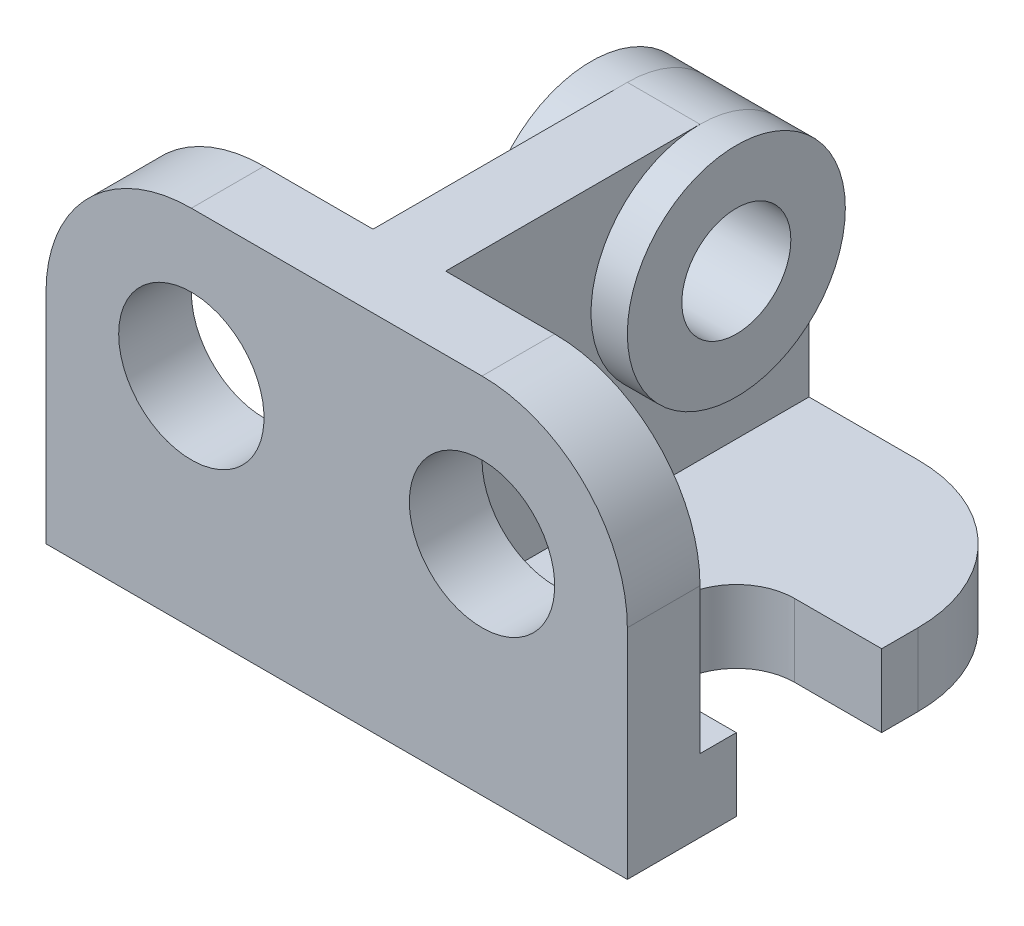
ISO-10303-21;
HEADER;
FILE_DESCRIPTION(('STEP AP214'),'2;1');
FILE_NAME('part.step','',(''),(''),'','','');
FILE_SCHEMA(('AUTOMOTIVE_DESIGN { 1 0 10303 214 1 1 1 1 }'));
ENDSEC;
DATA;
#1=APPLICATION_CONTEXT('core data for automotive mechanical design processes');
#2=APPLICATION_PROTOCOL_DEFINITION('international standard','automotive_design',2000,#1);
#3=PRODUCT_CONTEXT('',#1,'mechanical');
#4=PRODUCT('Part','Part','',(#3));
#5=PRODUCT_RELATED_PRODUCT_CATEGORY('part','',(#4));
#6=PRODUCT_DEFINITION_FORMATION('','',#4);
#7=PRODUCT_DEFINITION_CONTEXT('part definition',#1,'design');
#8=PRODUCT_DEFINITION('design','',#6,#7);
#9=PRODUCT_DEFINITION_SHAPE('','',#8);
#10=(LENGTH_UNIT() NAMED_UNIT(*) SI_UNIT(.MILLI.,.METRE.));
#11=(NAMED_UNIT(*) PLANE_ANGLE_UNIT() SI_UNIT($,.RADIAN.));
#12=(NAMED_UNIT(*) SI_UNIT($,.STERADIAN.) SOLID_ANGLE_UNIT());
#13=UNCERTAINTY_MEASURE_WITH_UNIT(LENGTH_MEASURE(1.E-05),#10,'distance_accuracy_value','');
#14=(GEOMETRIC_REPRESENTATION_CONTEXT(3) GLOBAL_UNCERTAINTY_ASSIGNED_CONTEXT((#13)) GLOBAL_UNIT_ASSIGNED_CONTEXT((#10,
#11,#12)) REPRESENTATION_CONTEXT('',''));
#15=CARTESIAN_POINT('',(0.,0.,0.));
#16=DIRECTION('',(0.,0.,1.));
#17=DIRECTION('',(1.,0.,0.));
#18=AXIS2_PLACEMENT_3D('',#15,#16,#17);
#19=CARTESIAN_POINT('',(4000.,0.,0.));
#20=DIRECTION('',(1.,0.,0.));
#21=DIRECTION('',(0.,0.,-1.));
#22=AXIS2_PLACEMENT_3D('',#19,#20,#21);
#23=PLANE('',#22);
#24=DIRECTION('',(0.,-1.,0.));
#25=VECTOR('',#24,1.);
#26=CARTESIAN_POINT('',(4000.,0.,1500.));
#27=LINE('',#26,#25);
#28=CARTESIAN_POINT('',(4000.,500.,1500.));
#29=VERTEX_POINT('',#28);
#30=CARTESIAN_POINT('',(4000.,-500.,1500.));
#31=VERTEX_POINT('',#30);
#32=EDGE_CURVE('E222',#29,#31,#27,.T.);
#33=ORIENTED_EDGE('',*,*,#32,.F.);
#34=DIRECTION('',(0.,0.,1.));
#35=VECTOR('',#34,1.);
#36=CARTESIAN_POINT('',(4000.,500.,2000.));
#37=LINE('',#36,#35);
#38=CARTESIAN_POINT('',(4000.,500.,2000.));
#39=VERTEX_POINT('',#38);
#40=EDGE_CURVE('E238',#29,#39,#37,.T.);
#41=ORIENTED_EDGE('',*,*,#40,.T.);
#42=DIRECTION('',(0.,1.,0.));
#43=VECTOR('',#42,1.);
#44=CARTESIAN_POINT('',(4000.,500.,2000.));
#45=LINE('',#44,#43);
#46=CARTESIAN_POINT('',(4000.,2500.,2000.));
#47=VERTEX_POINT('',#46);
#48=EDGE_CURVE('E240',#39,#47,#45,.T.);
#49=ORIENTED_EDGE('',*,*,#48,.T.);
#50=DIRECTION('',(0.,0.,1.));
#51=VECTOR('',#50,1.);
#52=CARTESIAN_POINT('',(4000.,2500.,3000.));
#53=LINE('',#52,#51);
#54=CARTESIAN_POINT('',(4000.,2500.,3000.));
#55=VERTEX_POINT('',#54);
#56=EDGE_CURVE('E285',#47,#55,#53,.T.);
#57=ORIENTED_EDGE('',*,*,#56,.T.);
#58=DIRECTION('',(0.,-1.,0.));
#59=VECTOR('',#58,1.);
#60=CARTESIAN_POINT('',(4000.,500.,3000.));
#61=LINE('',#60,#59);
#62=CARTESIAN_POINT('',(4000.,-500.,3000.));
#63=VERTEX_POINT('',#62);
#64=EDGE_CURVE('E241',#55,#63,#61,.T.);
#65=ORIENTED_EDGE('',*,*,#64,.T.);
#66=DIRECTION('',(0.,0.,-1.));
#67=VECTOR('',#66,1.);
#68=CARTESIAN_POINT('',(4000.,-500.,3000.));
#69=LINE('',#68,#67);
#70=EDGE_CURVE('E249',#63,#31,#69,.T.);
#71=ORIENTED_EDGE('',*,*,#70,.T.);
#72=EDGE_LOOP('',(#33,#41,#49,#57,#65,#71));
#73=FACE_BOUND('',#72,.T.);
#74=ADVANCED_FACE('F41',(#73),#23,.T.);
#75=CARTESIAN_POINT('',(-4000.,0.,0.));
#76=DIRECTION('',(1.,0.,0.));
#77=DIRECTION('',(0.,0.,-1.));
#78=AXIS2_PLACEMENT_3D('',#75,#76,#77);
#79=PLANE('',#78);
#80=DIRECTION('',(0.,0.,1.));
#81=VECTOR('',#80,1.);
#82=CARTESIAN_POINT('',(-4000.,500.,2000.));
#83=LINE('',#82,#81);
#84=CARTESIAN_POINT('',(-4000.,500.,1447.76070932594));
#85=VERTEX_POINT('',#84);
#86=CARTESIAN_POINT('',(-4000.,500.,2000.));
#87=VERTEX_POINT('',#86);
#88=EDGE_CURVE('E257',#85,#87,#83,.T.);
#89=ORIENTED_EDGE('',*,*,#88,.F.);
#90=DIRECTION('',(0.,-1.,0.));
#91=VECTOR('',#90,1.);
#92=CARTESIAN_POINT('',(-4000.,0.,1447.76070932594));
#93=LINE('',#92,#91);
#94=CARTESIAN_POINT('',(-4000.,-500.,1447.76070932594));
#95=VERTEX_POINT('',#94);
#96=EDGE_CURVE('E341',#85,#95,#93,.T.);
#97=ORIENTED_EDGE('',*,*,#96,.T.);
#98=DIRECTION('',(0.,0.,-1.));
#99=VECTOR('',#98,1.);
#100=CARTESIAN_POINT('',(-4000.,-500.,3000.));
#101=LINE('',#100,#99);
#102=CARTESIAN_POINT('',(-4000.,-500.,3000.));
#103=VERTEX_POINT('',#102);
#104=EDGE_CURVE('E243',#103,#95,#101,.T.);
#105=ORIENTED_EDGE('',*,*,#104,.F.);
#106=DIRECTION('',(0.,-1.,0.));
#107=VECTOR('',#106,1.);
#108=CARTESIAN_POINT('',(-4000.,500.,3000.));
#109=LINE('',#108,#107);
#110=CARTESIAN_POINT('',(-4000.,2500.,3000.));
#111=VERTEX_POINT('',#110);
#112=EDGE_CURVE('E263',#111,#103,#109,.T.);
#113=ORIENTED_EDGE('',*,*,#112,.F.);
#114=DIRECTION('',(0.,0.,1.));
#115=VECTOR('',#114,1.);
#116=CARTESIAN_POINT('',(-4000.,2500.,0.));
#117=LINE('',#116,#115);
#118=CARTESIAN_POINT('',(-4000.,2500.,2000.));
#119=VERTEX_POINT('',#118);
#120=EDGE_CURVE('E304',#111,#119,#117,.F.);
#121=ORIENTED_EDGE('',*,*,#120,.T.);
#122=DIRECTION('',(0.,1.,0.));
#123=VECTOR('',#122,1.);
#124=CARTESIAN_POINT('',(-4000.,500.,2000.));
#125=LINE('',#124,#123);
#126=EDGE_CURVE('E260',#87,#119,#125,.T.);
#127=ORIENTED_EDGE('',*,*,#126,.F.);
#128=EDGE_LOOP('',(#89,#97,#105,#113,#121,#127));
#129=FACE_BOUND('',#128,.T.);
#130=ADVANCED_FACE('F519',(#129),#79,.F.);
#131=CARTESIAN_POINT('',(500.,-500.,-3000.));
#132=DIRECTION('',(1.,0.,0.));
#133=DIRECTION('',(0.,0.,-1.));
#134=AXIS2_PLACEMENT_3D('',#131,#132,#133);
#135=PLANE('',#134);
#136=DIRECTION('',(0.,1.,0.));
#137=VECTOR('',#136,1.);
#138=CARTESIAN_POINT('',(500.,-500.,-3000.));
#139=LINE('',#138,#137);
#140=CARTESIAN_POINT('',(500.,500.,-3000.));
#141=VERTEX_POINT('',#140);
#142=CARTESIAN_POINT('',(500.,3000.,-3000.));
#143=VERTEX_POINT('',#142);
#144=EDGE_CURVE('E431',#141,#143,#139,.T.);
#145=ORIENTED_EDGE('',*,*,#144,.T.);
#146=CARTESIAN_POINT('',(500.,3000.,-1500.));
#147=DIRECTION('',(1.,0.,0.));
#148=DIRECTION('',(0.,0.,-1.));
#149=AXIS2_PLACEMENT_3D('',#146,#147,#148);
#150=CIRCLE('',#149,1500.);
#151=CARTESIAN_POINT('',(500.,4500.,-1500.));
#152=VERTEX_POINT('',#151);
#153=EDGE_CURVE('E335',#143,#152,#150,.F.);
#154=ORIENTED_EDGE('',*,*,#153,.T.);
#155=DIRECTION('',(0.,0.,-1.));
#156=VECTOR('',#155,1.);
#157=CARTESIAN_POINT('',(500.,4500.,-3000.));
#158=LINE('',#157,#156);
#159=CARTESIAN_POINT('',(500.,4500.,2000.));
#160=VERTEX_POINT('',#159);
#161=EDGE_CURVE('E426',#160,#152,#158,.T.);
#162=ORIENTED_EDGE('',*,*,#161,.F.);
#163=DIRECTION('',(0.,1.,0.));
#164=VECTOR('',#163,1.);
#165=CARTESIAN_POINT('',(500.,500.,2000.));
#166=LINE('',#165,#164);
#167=CARTESIAN_POINT('',(500.,500.,2000.));
#168=VERTEX_POINT('',#167);
#169=EDGE_CURVE('E434',#168,#160,#166,.T.);
#170=ORIENTED_EDGE('',*,*,#169,.F.);
#171=DIRECTION('',(0.,0.,1.));
#172=VECTOR('',#171,1.);
#173=CARTESIAN_POINT('',(500.,500.,2000.));
#174=LINE('',#173,#172);
#175=EDGE_CURVE('E439',#141,#168,#174,.T.);
#176=ORIENTED_EDGE('',*,*,#175,.F.);
#177=EDGE_LOOP('',(#145,#154,#162,#170,#176));
#178=FACE_BOUND('',#177,.T.);
#179=ADVANCED_FACE('F555',(#178),#135,.T.);
#180=CARTESIAN_POINT('',(4000.,500.,2000.));
#181=DIRECTION('',(0.,-1.,0.));
#182=DIRECTION('',(0.,0.,-1.));
#183=AXIS2_PLACEMENT_3D('',#180,#181,#182);
#184=PLANE('',#183);
#185=DIRECTION('',(0.,0.,-1.));
#186=VECTOR('',#185,1.);
#187=CARTESIAN_POINT('',(-2000.,500.,447.760709325942));
#188=LINE('',#187,#186);
#189=CARTESIAN_POINT('',(-2000.,500.,647.760709325942));
#190=VERTEX_POINT('',#189);
#191=CARTESIAN_POINT('',(-2000.,500.,247.760709325942));
#192=VERTEX_POINT('',#191);
#193=EDGE_CURVE('E400',#190,#192,#188,.T.);
#194=ORIENTED_EDGE('',*,*,#193,.F.);
#195=CARTESIAN_POINT('',(-2800.,500.,647.760709325942));
#196=DIRECTION('',(0.,-1.,0.));
#197=DIRECTION('',(0.,0.,-1.));
#198=AXIS2_PLACEMENT_3D('',#195,#196,#197);
#199=CIRCLE('',#198,800.);
#200=CARTESIAN_POINT('',(-2800.,500.,1447.76070932594));
#201=VERTEX_POINT('',#200);
#202=EDGE_CURVE('E355',#190,#201,#199,.T.);
#203=ORIENTED_EDGE('',*,*,#202,.T.);
#204=DIRECTION('',(1.,0.,0.));
#205=VECTOR('',#204,1.);
#206=CARTESIAN_POINT('',(-5200.,500.,1447.76070932594));
#207=LINE('',#206,#205);
#208=EDGE_CURVE('E405',#85,#201,#207,.T.);
#209=ORIENTED_EDGE('',*,*,#208,.F.);
#210=ORIENTED_EDGE('',*,*,#88,.T.);
#211=DIRECTION('',(-1.,0.,0.));
#212=VECTOR('',#211,1.);
#213=CARTESIAN_POINT('',(4000.,500.,2000.));
#214=LINE('',#213,#212);
#215=CARTESIAN_POINT('',(-500.,500.,2000.));
#216=VERTEX_POINT('',#215);
#217=EDGE_CURVE('E276',#216,#87,#214,.T.);
#218=ORIENTED_EDGE('',*,*,#217,.F.);
#219=DIRECTION('',(0.,0.,-1.));
#220=VECTOR('',#219,1.);
#221=CARTESIAN_POINT('',(-500.,500.,2000.));
#222=LINE('',#221,#220);
#223=CARTESIAN_POINT('',(-500.,500.,-3000.));
#224=VERTEX_POINT('',#223);
#225=EDGE_CURVE('E447',#216,#224,#222,.T.);
#226=ORIENTED_EDGE('',*,*,#225,.T.);
#227=DIRECTION('',(-1.,0.,0.));
#228=VECTOR('',#227,1.);
#229=CARTESIAN_POINT('',(4000.,500.,-3000.));
#230=LINE('',#229,#228);
#231=CARTESIAN_POINT('',(-2000.,500.,-3000.));
#232=VERTEX_POINT('',#231);
#233=EDGE_CURVE('E279',#224,#232,#230,.T.);
#234=ORIENTED_EDGE('',*,*,#233,.T.);
#235=CARTESIAN_POINT('',(-2000.,500.,-1000.));
#236=DIRECTION('',(0.,-1.,0.));
#237=DIRECTION('',(0.,0.,-1.));
#238=AXIS2_PLACEMENT_3D('',#235,#236,#237);
#239=CIRCLE('',#238,2000.);
#240=CARTESIAN_POINT('',(-4000.,500.,-1000.));
#241=VERTEX_POINT('',#240);
#242=EDGE_CURVE('E321',#232,#241,#239,.F.);
#243=ORIENTED_EDGE('',*,*,#242,.T.);
#244=CARTESIAN_POINT('',(-4000.,500.,-552.239290674058));
#245=VERTEX_POINT('',#244);
#246=EDGE_CURVE('E251',#241,#245,#83,.T.);
#247=ORIENTED_EDGE('',*,*,#246,.T.);
#248=DIRECTION('',(-1.,0.,0.));
#249=VECTOR('',#248,1.);
#250=CARTESIAN_POINT('',(-5200.,500.,-552.239290674058));
#251=LINE('',#250,#249);
#252=CARTESIAN_POINT('',(-2800.,500.,-552.239290674058));
#253=VERTEX_POINT('',#252);
#254=EDGE_CURVE('E399',#253,#245,#251,.T.);
#255=ORIENTED_EDGE('',*,*,#254,.F.);
#256=CARTESIAN_POINT('',(-2800.,500.,247.760709325942));
#257=DIRECTION('',(0.,-1.,0.));
#258=DIRECTION('',(0.,0.,-1.));
#259=AXIS2_PLACEMENT_3D('',#256,#257,#258);
#260=CIRCLE('',#259,800.);
#261=EDGE_CURVE('E363',#253,#192,#260,.T.);
#262=ORIENTED_EDGE('',*,*,#261,.T.);
#263=EDGE_LOOP('',(#194,#203,#209,#210,#218,#226,#234,#243,#247,#255,#262));
#264=FACE_BOUND('',#263,.T.);
#265=ADVANCED_FACE('F461',(#264),#184,.F.);
#266=CARTESIAN_POINT('',(4000.,500.,2000.));
#267=DIRECTION('',(0.,0.,1.));
#268=DIRECTION('',(1.,0.,0.));
#269=AXIS2_PLACEMENT_3D('',#266,#267,#268);
#270=PLANE('',#269);
#271=CARTESIAN_POINT('',(-2000.,2500.,2000.));
#272=DIRECTION('',(0.,0.,-1.));
#273=DIRECTION('',(-1.,0.,0.));
#274=AXIS2_PLACEMENT_3D('',#271,#272,#273);
#275=CIRCLE('',#274,1000.);
#276=CARTESIAN_POINT('',(-3000.,2500.,2000.));
#277=VERTEX_POINT('',#276);
#278=EDGE_CURVE('E244',#277,#277,#275,.T.);
#279=ORIENTED_EDGE('',*,*,#278,.F.);
#280=EDGE_LOOP('',(#279));
#281=FACE_BOUND('',#280,.T.);
#282=DIRECTION('',(-1.,0.,0.));
#283=VECTOR('',#282,1.);
#284=CARTESIAN_POINT('',(4000.,4500.,2000.));
#285=LINE('',#284,#283);
#286=CARTESIAN_POINT('',(-500.,4500.,2000.));
#287=VERTEX_POINT('',#286);
#288=CARTESIAN_POINT('',(-2000.,4500.,2000.));
#289=VERTEX_POINT('',#288);
#290=EDGE_CURVE('E275',#287,#289,#285,.T.);
#291=ORIENTED_EDGE('',*,*,#290,.F.);
#292=DIRECTION('',(0.,-1.,0.));
#293=VECTOR('',#292,1.);
#294=CARTESIAN_POINT('',(-500.,500.,2000.));
#295=LINE('',#294,#293);
#296=EDGE_CURVE('E442',#287,#216,#295,.T.);
#297=ORIENTED_EDGE('',*,*,#296,.T.);
#298=ORIENTED_EDGE('',*,*,#217,.T.);
#299=ORIENTED_EDGE('',*,*,#126,.T.);
#300=CARTESIAN_POINT('',(-2000.,2500.,2000.));
#301=DIRECTION('',(0.,0.,1.));
#302=DIRECTION('',(1.,0.,0.));
#303=AXIS2_PLACEMENT_3D('',#300,#301,#302);
#304=CIRCLE('',#303,2000.);
#305=EDGE_CURVE('E310',#119,#289,#304,.F.);
#306=ORIENTED_EDGE('',*,*,#305,.T.);
#307=EDGE_LOOP('',(#291,#297,#298,#299,#306));
#308=FACE_BOUND('',#307,.T.);
#309=ADVANCED_FACE('F459',(#281,#308),#270,.F.);
#310=CARTESIAN_POINT('',(4000.,500.,-3000.));
#311=DIRECTION('',(0.,0.,1.));
#312=DIRECTION('',(1.,0.,0.));
#313=AXIS2_PLACEMENT_3D('',#310,#311,#312);
#314=PLANE('',#313);
#315=DIRECTION('',(0.,1.,0.));
#316=VECTOR('',#315,1.);
#317=CARTESIAN_POINT('',(-500.,-500.,-3000.));
#318=LINE('',#317,#316);
#319=CARTESIAN_POINT('',(-500.,3000.,-3000.));
#320=VERTEX_POINT('',#319);
#321=EDGE_CURVE('E435',#224,#320,#318,.T.);
#322=ORIENTED_EDGE('',*,*,#321,.T.);
#323=DIRECTION('',(-1.,0.,0.));
#324=VECTOR('',#323,1.);
#325=CARTESIAN_POINT('',(4000.,3000.,-3000.));
#326=LINE('',#325,#324);
#327=EDGE_CURVE('E337',#320,#143,#326,.F.);
#328=ORIENTED_EDGE('',*,*,#327,.T.);
#329=ORIENTED_EDGE('',*,*,#144,.F.);
#330=CARTESIAN_POINT('',(2000.,500.,-3000.));
#331=VERTEX_POINT('',#330);
#332=EDGE_CURVE('E283',#331,#141,#230,.T.);
#333=ORIENTED_EDGE('',*,*,#332,.F.);
#334=DIRECTION('',(0.,1.,0.));
#335=VECTOR('',#334,1.);
#336=CARTESIAN_POINT('',(2000.,-500.,-3000.));
#337=LINE('',#336,#335);
#338=CARTESIAN_POINT('',(2000.,-500.,-3000.));
#339=VERTEX_POINT('',#338);
#340=EDGE_CURVE('E312',#331,#339,#337,.F.);
#341=ORIENTED_EDGE('',*,*,#340,.T.);
#342=DIRECTION('',(-1.,0.,0.));
#343=VECTOR('',#342,1.);
#344=CARTESIAN_POINT('',(4000.,-500.,-3000.));
#345=LINE('',#344,#343);
#346=CARTESIAN_POINT('',(-2000.,-500.,-3000.));
#347=VERTEX_POINT('',#346);
#348=EDGE_CURVE('E254',#339,#347,#345,.T.);
#349=ORIENTED_EDGE('',*,*,#348,.T.);
#350=DIRECTION('',(0.,1.,0.));
#351=VECTOR('',#350,1.);
#352=CARTESIAN_POINT('',(-2000.,500.,-3000.));
#353=LINE('',#352,#351);
#354=EDGE_CURVE('E319',#347,#232,#353,.T.);
#355=ORIENTED_EDGE('',*,*,#354,.T.);
#356=ORIENTED_EDGE('',*,*,#233,.F.);
#357=EDGE_LOOP('',(#322,#328,#329,#333,#341,#349,#355,#356));
#358=FACE_BOUND('',#357,.T.);
#359=ADVANCED_FACE('F456',(#358),#314,.F.);
#360=ORIENTED_EDGE('',*,*,#40,.F.);
#361=DIRECTION('',(1.,0.,0.));
#362=VECTOR('',#361,1.);
#363=CARTESIAN_POINT('',(2000.,500.,1500.));
#364=LINE('',#363,#362);
#365=CARTESIAN_POINT('',(2800.,500.,1500.));
#366=VERTEX_POINT('',#365);
#367=EDGE_CURVE('E389',#366,#29,#364,.T.);
#368=ORIENTED_EDGE('',*,*,#367,.F.);
#369=CARTESIAN_POINT('',(2800.,500.,700.));
#370=DIRECTION('',(0.,-1.,0.));
#371=DIRECTION('',(0.,0.,-1.));
#372=AXIS2_PLACEMENT_3D('',#369,#370,#371);
#373=CIRCLE('',#372,800.);
#374=CARTESIAN_POINT('',(2000.,500.,700.));
#375=VERTEX_POINT('',#374);
#376=EDGE_CURVE('E372',#366,#375,#373,.T.);
#377=ORIENTED_EDGE('',*,*,#376,.T.);
#378=DIRECTION('',(0.,0.,1.));
#379=VECTOR('',#378,1.);
#380=CARTESIAN_POINT('',(2000.,500.,-500.000000000001));
#381=LINE('',#380,#379);
#382=CARTESIAN_POINT('',(2000.,500.,299.999999999999));
#383=VERTEX_POINT('',#382);
#384=EDGE_CURVE('E233',#383,#375,#381,.T.);
#385=ORIENTED_EDGE('',*,*,#384,.F.);
#386=CARTESIAN_POINT('',(2800.,500.,299.999999999999));
#387=DIRECTION('',(0.,-1.,0.));
#388=DIRECTION('',(0.,0.,-1.));
#389=AXIS2_PLACEMENT_3D('',#386,#387,#388);
#390=CIRCLE('',#389,800.);
#391=CARTESIAN_POINT('',(2800.,500.,-500.000000000001));
#392=VERTEX_POINT('',#391);
#393=EDGE_CURVE('E47',#383,#392,#390,.T.);
#394=ORIENTED_EDGE('',*,*,#393,.T.);
#395=DIRECTION('',(-1.,0.,0.));
#396=VECTOR('',#395,1.);
#397=CARTESIAN_POINT('',(2000.,500.,-500.000000000001));
#398=LINE('',#397,#396);
#399=CARTESIAN_POINT('',(4000.,500.,-500.000000000001));
#400=VERTEX_POINT('',#399);
#401=EDGE_CURVE('E220',#400,#392,#398,.T.);
#402=ORIENTED_EDGE('',*,*,#401,.F.);
#403=CARTESIAN_POINT('',(4000.,500.,-1000.));
#404=VERTEX_POINT('',#403);
#405=EDGE_CURVE('E229',#404,#400,#37,.T.);
#406=ORIENTED_EDGE('',*,*,#405,.F.);
#407=CARTESIAN_POINT('',(2000.,500.,-1000.));
#408=DIRECTION('',(0.,-1.,0.));
#409=DIRECTION('',(0.,0.,-1.));
#410=AXIS2_PLACEMENT_3D('',#407,#408,#409);
#411=CIRCLE('',#410,2000.);
#412=EDGE_CURVE('E311',#404,#331,#411,.F.);
#413=ORIENTED_EDGE('',*,*,#412,.T.);
#414=ORIENTED_EDGE('',*,*,#332,.T.);
#415=ORIENTED_EDGE('',*,*,#175,.T.);
#416=EDGE_CURVE('E280',#39,#168,#214,.T.);
#417=ORIENTED_EDGE('',*,*,#416,.F.);
#418=EDGE_LOOP('',(#360,#368,#377,#385,#394,#402,#406,#413,#414,#415,#417));
#419=FACE_BOUND('',#418,.T.);
#420=ADVANCED_FACE('F230',(#419),#184,.F.);
#421=CARTESIAN_POINT('',(2000.,2500.,2000.));
#422=DIRECTION('',(0.,0.,-1.));
#423=DIRECTION('',(-1.,0.,0.));
#424=AXIS2_PLACEMENT_3D('',#421,#422,#423);
#425=CIRCLE('',#424,1000.);
#426=CARTESIAN_POINT('',(1000.,2500.,2000.));
#427=VERTEX_POINT('',#426);
#428=EDGE_CURVE('E287',#427,#427,#425,.T.);
#429=ORIENTED_EDGE('',*,*,#428,.F.);
#430=EDGE_LOOP('',(#429));
#431=FACE_BOUND('',#430,.T.);
#432=ORIENTED_EDGE('',*,*,#416,.T.);
#433=ORIENTED_EDGE('',*,*,#169,.T.);
#434=CARTESIAN_POINT('',(2000.,4500.,2000.));
#435=VERTEX_POINT('',#434);
#436=EDGE_CURVE('E271',#435,#160,#285,.T.);
#437=ORIENTED_EDGE('',*,*,#436,.F.);
#438=CARTESIAN_POINT('',(2000.,2500.,2000.));
#439=DIRECTION('',(0.,0.,1.));
#440=DIRECTION('',(1.,0.,0.));
#441=AXIS2_PLACEMENT_3D('',#438,#439,#440);
#442=CIRCLE('',#441,2000.);
#443=EDGE_CURVE('E296',#435,#47,#442,.F.);
#444=ORIENTED_EDGE('',*,*,#443,.T.);
#445=ORIENTED_EDGE('',*,*,#48,.F.);
#446=EDGE_LOOP('',(#432,#433,#437,#444,#445));
#447=FACE_BOUND('',#446,.T.);
#448=ADVANCED_FACE('F463',(#431,#447),#270,.F.);
#449=CARTESIAN_POINT('',(4000.,4500.,3000.));
#450=DIRECTION('',(0.,-1.,0.));
#451=DIRECTION('',(0.,0.,-1.));
#452=AXIS2_PLACEMENT_3D('',#449,#450,#451);
#453=PLANE('',#452);
#454=ORIENTED_EDGE('',*,*,#161,.T.);
#455=DIRECTION('',(-1.,0.,0.));
#456=VECTOR('',#455,1.);
#457=CARTESIAN_POINT('',(4000.,4500.,-1500.));
#458=LINE('',#457,#456);
#459=CARTESIAN_POINT('',(-500.,4500.,-1500.));
#460=VERTEX_POINT('',#459);
#461=EDGE_CURVE('E333',#152,#460,#458,.T.);
#462=ORIENTED_EDGE('',*,*,#461,.T.);
#463=DIRECTION('',(0.,0.,1.));
#464=VECTOR('',#463,1.);
#465=CARTESIAN_POINT('',(-500.,4500.,-3000.));
#466=LINE('',#465,#464);
#467=EDGE_CURVE('E428',#460,#287,#466,.T.);
#468=ORIENTED_EDGE('',*,*,#467,.T.);
#469=ORIENTED_EDGE('',*,*,#290,.T.);
#470=DIRECTION('',(0.,0.,1.));
#471=VECTOR('',#470,1.);
#472=CARTESIAN_POINT('',(-2000.,4500.,3000.));
#473=LINE('',#472,#471);
#474=CARTESIAN_POINT('',(-2000.,4500.,3000.));
#475=VERTEX_POINT('',#474);
#476=EDGE_CURVE('E297',#289,#475,#473,.T.);
#477=ORIENTED_EDGE('',*,*,#476,.T.);
#478=DIRECTION('',(-1.,0.,0.));
#479=VECTOR('',#478,1.);
#480=CARTESIAN_POINT('',(4000.,4500.,3000.));
#481=LINE('',#480,#479);
#482=CARTESIAN_POINT('',(2000.,4500.,3000.));
#483=VERTEX_POINT('',#482);
#484=EDGE_CURVE('E269',#483,#475,#481,.T.);
#485=ORIENTED_EDGE('',*,*,#484,.F.);
#486=DIRECTION('',(0.,0.,1.));
#487=VECTOR('',#486,1.);
#488=CARTESIAN_POINT('',(2000.,4500.,2000.));
#489=LINE('',#488,#487);
#490=EDGE_CURVE('E298',#483,#435,#489,.F.);
#491=ORIENTED_EDGE('',*,*,#490,.T.);
#492=ORIENTED_EDGE('',*,*,#436,.T.);
#493=EDGE_LOOP('',(#454,#462,#468,#469,#477,#485,#491,#492));
#494=FACE_BOUND('',#493,.T.);
#495=ADVANCED_FACE('F471',(#494),#453,.F.);
#496=CARTESIAN_POINT('',(4000.,500.,3000.));
#497=DIRECTION('',(0.,0.,-1.));
#498=DIRECTION('',(-1.,0.,0.));
#499=AXIS2_PLACEMENT_3D('',#496,#497,#498);
#500=PLANE('',#499);
#501=CARTESIAN_POINT('',(2000.,2500.,3000.));
#502=DIRECTION('',(0.,0.,-1.));
#503=DIRECTION('',(-1.,0.,0.));
#504=AXIS2_PLACEMENT_3D('',#501,#502,#503);
#505=CIRCLE('',#504,1000.);
#506=CARTESIAN_POINT('',(1000.,2500.,3000.));
#507=VERTEX_POINT('',#506);
#508=EDGE_CURVE('E288',#507,#507,#505,.T.);
#509=ORIENTED_EDGE('',*,*,#508,.T.);
#510=EDGE_LOOP('',(#509));
#511=FACE_BOUND('',#510,.T.);
#512=ORIENTED_EDGE('',*,*,#484,.T.);
#513=CARTESIAN_POINT('',(-2000.,2500.,3000.));
#514=DIRECTION('',(0.,0.,-1.));
#515=DIRECTION('',(-1.,0.,0.));
#516=AXIS2_PLACEMENT_3D('',#513,#514,#515);
#517=CIRCLE('',#516,2000.);
#518=EDGE_CURVE('E303',#475,#111,#517,.F.);
#519=ORIENTED_EDGE('',*,*,#518,.T.);
#520=ORIENTED_EDGE('',*,*,#112,.T.);
#521=DIRECTION('',(-1.,0.,0.));
#522=VECTOR('',#521,1.);
#523=CARTESIAN_POINT('',(4000.,-500.,3000.));
#524=LINE('',#523,#522);
#525=EDGE_CURVE('E268',#63,#103,#524,.T.);
#526=ORIENTED_EDGE('',*,*,#525,.F.);
#527=ORIENTED_EDGE('',*,*,#64,.F.);
#528=CARTESIAN_POINT('',(2000.,2500.,3000.));
#529=DIRECTION('',(0.,0.,-1.));
#530=DIRECTION('',(-1.,0.,0.));
#531=AXIS2_PLACEMENT_3D('',#528,#529,#530);
#532=CIRCLE('',#531,2000.);
#533=EDGE_CURVE('E295',#55,#483,#532,.F.);
#534=ORIENTED_EDGE('',*,*,#533,.T.);
#535=EDGE_LOOP('',(#512,#519,#520,#526,#527,#534));
#536=FACE_BOUND('',#535,.T.);
#537=CARTESIAN_POINT('',(-2000.,2500.,3000.));
#538=DIRECTION('',(0.,0.,-1.));
#539=DIRECTION('',(-1.,0.,0.));
#540=AXIS2_PLACEMENT_3D('',#537,#538,#539);
#541=CIRCLE('',#540,1000.);
#542=CARTESIAN_POINT('',(-3000.,2500.,3000.));
#543=VERTEX_POINT('',#542);
#544=EDGE_CURVE('E281',#543,#543,#541,.T.);
#545=ORIENTED_EDGE('',*,*,#544,.T.);
#546=EDGE_LOOP('',(#545));
#547=FACE_BOUND('',#546,.T.);
#548=ADVANCED_FACE('F530',(#511,#536,#547),#500,.F.);
#549=CARTESIAN_POINT('',(4000.,-500.,3000.));
#550=DIRECTION('',(0.,1.,0.));
#551=DIRECTION('',(0.,0.,1.));
#552=AXIS2_PLACEMENT_3D('',#549,#550,#551);
#553=PLANE('',#552);
#554=DIRECTION('',(-1.,0.,0.));
#555=VECTOR('',#554,1.);
#556=CARTESIAN_POINT('',(4000.,-500.,-500.));
#557=LINE('',#556,#555);
#558=CARTESIAN_POINT('',(4000.,-500.,-500.));
#559=VERTEX_POINT('',#558);
#560=CARTESIAN_POINT('',(2800.,-500.,-500.));
#561=VERTEX_POINT('',#560);
#562=EDGE_CURVE('E216',#559,#561,#557,.T.);
#563=ORIENTED_EDGE('',*,*,#562,.T.);
#564=CARTESIAN_POINT('',(2800.,-500.,299.999999999999));
#565=DIRECTION('',(0.,1.,0.));
#566=DIRECTION('',(0.,0.,1.));
#567=AXIS2_PLACEMENT_3D('',#564,#565,#566);
#568=CIRCLE('',#567,800.);
#569=CARTESIAN_POINT('',(2000.,-500.,299.999999999999));
#570=VERTEX_POINT('',#569);
#571=EDGE_CURVE('E11',#561,#570,#568,.T.);
#572=ORIENTED_EDGE('',*,*,#571,.T.);
#573=DIRECTION('',(0.,0.,1.));
#574=VECTOR('',#573,1.);
#575=CARTESIAN_POINT('',(2000.,-500.,3000.));
#576=LINE('',#575,#574);
#577=CARTESIAN_POINT('',(2000.,-500.,700.));
#578=VERTEX_POINT('',#577);
#579=EDGE_CURVE('E366',#570,#578,#576,.T.);
#580=ORIENTED_EDGE('',*,*,#579,.T.);
#581=CARTESIAN_POINT('',(2800.,-500.,700.));
#582=DIRECTION('',(0.,1.,0.));
#583=DIRECTION('',(0.,0.,1.));
#584=AXIS2_PLACEMENT_3D('',#581,#582,#583);
#585=CIRCLE('',#584,800.);
#586=CARTESIAN_POINT('',(2800.,-500.,1500.));
#587=VERTEX_POINT('',#586);
#588=EDGE_CURVE('E380',#578,#587,#585,.T.);
#589=ORIENTED_EDGE('',*,*,#588,.T.);
#590=DIRECTION('',(1.,0.,0.));
#591=VECTOR('',#590,1.);
#592=CARTESIAN_POINT('',(4000.,-500.,1500.));
#593=LINE('',#592,#591);
#594=EDGE_CURVE('E391',#587,#31,#593,.T.);
#595=ORIENTED_EDGE('',*,*,#594,.T.);
#596=ORIENTED_EDGE('',*,*,#70,.F.);
#597=ORIENTED_EDGE('',*,*,#525,.T.);
#598=ORIENTED_EDGE('',*,*,#104,.T.);
#599=DIRECTION('',(1.,0.,0.));
#600=VECTOR('',#599,1.);
#601=CARTESIAN_POINT('',(4000.,-500.,1447.76070932594));
#602=LINE('',#601,#600);
#603=CARTESIAN_POINT('',(-2800.,-500.,1447.76070932594));
#604=VERTEX_POINT('',#603);
#605=EDGE_CURVE('E410',#95,#604,#602,.T.);
#606=ORIENTED_EDGE('',*,*,#605,.T.);
#607=CARTESIAN_POINT('',(-2800.,-500.,647.760709325942));
#608=DIRECTION('',(0.,1.,0.));
#609=DIRECTION('',(0.,0.,1.));
#610=AXIS2_PLACEMENT_3D('',#607,#608,#609);
#611=CIRCLE('',#610,800.);
#612=CARTESIAN_POINT('',(-2000.,-500.,647.760709325941));
#613=VERTEX_POINT('',#612);
#614=EDGE_CURVE('E352',#604,#613,#611,.T.);
#615=ORIENTED_EDGE('',*,*,#614,.T.);
#616=DIRECTION('',(0.,0.,-1.));
#617=VECTOR('',#616,1.);
#618=CARTESIAN_POINT('',(-2000.,-500.,3000.));
#619=LINE('',#618,#617);
#620=CARTESIAN_POINT('',(-2000.,-500.,247.760709325942));
#621=VERTEX_POINT('',#620);
#622=EDGE_CURVE('E343',#613,#621,#619,.T.);
#623=ORIENTED_EDGE('',*,*,#622,.T.);
#624=CARTESIAN_POINT('',(-2800.,-500.,247.760709325942));
#625=DIRECTION('',(0.,1.,0.));
#626=DIRECTION('',(0.,0.,1.));
#627=AXIS2_PLACEMENT_3D('',#624,#625,#626);
#628=CIRCLE('',#627,800.);
#629=CARTESIAN_POINT('',(-2800.,-500.,-552.239290674058));
#630=VERTEX_POINT('',#629);
#631=EDGE_CURVE('E224',#621,#630,#628,.T.);
#632=ORIENTED_EDGE('',*,*,#631,.T.);
#633=DIRECTION('',(-1.,0.,0.));
#634=VECTOR('',#633,1.);
#635=CARTESIAN_POINT('',(4000.,-500.,-552.239290674058));
#636=LINE('',#635,#634);
#637=CARTESIAN_POINT('',(-4000.,-500.,-552.239290674058));
#638=VERTEX_POINT('',#637);
#639=EDGE_CURVE('E403',#630,#638,#636,.T.);
#640=ORIENTED_EDGE('',*,*,#639,.T.);
#641=CARTESIAN_POINT('',(-4000.,-500.,-1000.));
#642=VERTEX_POINT('',#641);
#643=EDGE_CURVE('E265',#638,#642,#101,.T.);
#644=ORIENTED_EDGE('',*,*,#643,.T.);
#645=CARTESIAN_POINT('',(-2000.,-500.,-1000.));
#646=DIRECTION('',(0.,1.,0.));
#647=DIRECTION('',(0.,0.,1.));
#648=AXIS2_PLACEMENT_3D('',#645,#646,#647);
#649=CIRCLE('',#648,2000.);
#650=EDGE_CURVE('E328',#642,#347,#649,.F.);
#651=ORIENTED_EDGE('',*,*,#650,.T.);
#652=ORIENTED_EDGE('',*,*,#348,.F.);
#653=CARTESIAN_POINT('',(2000.,-500.,-1000.));
#654=DIRECTION('',(0.,1.,0.));
#655=DIRECTION('',(0.,0.,1.));
#656=AXIS2_PLACEMENT_3D('',#653,#654,#655);
#657=CIRCLE('',#656,2000.);
#658=CARTESIAN_POINT('',(4000.,-500.,-1000.));
#659=VERTEX_POINT('',#658);
#660=EDGE_CURVE('E314',#339,#659,#657,.F.);
#661=ORIENTED_EDGE('',*,*,#660,.T.);
#662=EDGE_CURVE('E248',#559,#659,#69,.T.);
#663=ORIENTED_EDGE('',*,*,#662,.F.);
#664=EDGE_LOOP('',(#563,#572,#580,#589,#595,#596,#597,#598,#606,#615,#623,#632,#640,#644,#651,
#652,#661,#663));
#665=FACE_BOUND('',#664,.T.);
#666=ADVANCED_FACE('F508',(#665),#553,.F.);
#667=DIRECTION('',(0.,1.,0.));
#668=VECTOR('',#667,1.);
#669=CARTESIAN_POINT('',(4000.,0.,-500.000000000001));
#670=LINE('',#669,#668);
#671=EDGE_CURVE('E219',#559,#400,#670,.T.);
#672=ORIENTED_EDGE('',*,*,#671,.F.);
#673=ORIENTED_EDGE('',*,*,#662,.T.);
#674=DIRECTION('',(0.,1.,0.));
#675=VECTOR('',#674,1.);
#676=CARTESIAN_POINT('',(4000.,500.,-1000.));
#677=LINE('',#676,#675);
#678=EDGE_CURVE('E236',#659,#404,#677,.T.);
#679=ORIENTED_EDGE('',*,*,#678,.T.);
#680=ORIENTED_EDGE('',*,*,#405,.T.);
#681=EDGE_LOOP('',(#672,#673,#679,#680));
#682=FACE_BOUND('',#681,.T.);
#683=ADVANCED_FACE('F234',(#682),#23,.T.);
#684=ORIENTED_EDGE('',*,*,#643,.F.);
#685=DIRECTION('',(0.,1.,0.));
#686=VECTOR('',#685,1.);
#687=CARTESIAN_POINT('',(-4000.,0.,-552.239290674058));
#688=LINE('',#687,#686);
#689=EDGE_CURVE('E336',#638,#245,#688,.T.);
#690=ORIENTED_EDGE('',*,*,#689,.T.);
#691=ORIENTED_EDGE('',*,*,#246,.F.);
#692=DIRECTION('',(0.,1.,0.));
#693=VECTOR('',#692,1.);
#694=CARTESIAN_POINT('',(-4000.,0.,-1000.));
#695=LINE('',#694,#693);
#696=EDGE_CURVE('E322',#241,#642,#695,.F.);
#697=ORIENTED_EDGE('',*,*,#696,.T.);
#698=EDGE_LOOP('',(#684,#690,#691,#697));
#699=FACE_BOUND('',#698,.T.);
#700=ADVANCED_FACE('F494',(#699),#79,.F.);
#701=CARTESIAN_POINT('',(-2000.,2500.,10000.));
#702=DIRECTION('',(0.,0.,-1.));
#703=DIRECTION('',(-1.,0.,0.));
#704=AXIS2_PLACEMENT_3D('',#701,#702,#703);
#705=CYLINDRICAL_SURFACE('',#704,1000.);
#706=ORIENTED_EDGE('',*,*,#278,.T.);
#707=EDGE_LOOP('',(#706));
#708=FACE_BOUND('',#707,.T.);
#709=ORIENTED_EDGE('',*,*,#544,.F.);
#710=EDGE_LOOP('',(#709));
#711=FACE_BOUND('',#710,.T.);
#712=ADVANCED_FACE('F453',(#708,#711),#705,.F.);
#713=CARTESIAN_POINT('',(2000.,2500.,10000.));
#714=DIRECTION('',(0.,0.,-1.));
#715=DIRECTION('',(-1.,0.,0.));
#716=AXIS2_PLACEMENT_3D('',#713,#714,#715);
#717=CYLINDRICAL_SURFACE('',#716,1000.);
#718=ORIENTED_EDGE('',*,*,#428,.T.);
#719=EDGE_LOOP('',(#718));
#720=FACE_BOUND('',#719,.T.);
#721=ORIENTED_EDGE('',*,*,#508,.F.);
#722=EDGE_LOOP('',(#721));
#723=FACE_BOUND('',#722,.T.);
#724=ADVANCED_FACE('F542',(#720,#723),#717,.F.);
#725=CARTESIAN_POINT('',(2000.,2500.,0.));
#726=DIRECTION('',(0.,0.,-1.));
#727=DIRECTION('',(-1.,0.,0.));
#728=AXIS2_PLACEMENT_3D('',#725,#726,#727);
#729=CYLINDRICAL_SURFACE('',#728,2000.);
#730=ORIENTED_EDGE('',*,*,#443,.F.);
#731=ORIENTED_EDGE('',*,*,#490,.F.);
#732=ORIENTED_EDGE('',*,*,#533,.F.);
#733=ORIENTED_EDGE('',*,*,#56,.F.);
#734=EDGE_LOOP('',(#730,#731,#732,#733));
#735=FACE_BOUND('',#734,.T.);
#736=ADVANCED_FACE('F533',(#735),#729,.T.);
#737=CARTESIAN_POINT('',(-2000.,2500.,3000.));
#738=DIRECTION('',(0.,0.,1.));
#739=DIRECTION('',(1.,0.,0.));
#740=AXIS2_PLACEMENT_3D('',#737,#738,#739);
#741=CYLINDRICAL_SURFACE('',#740,2000.);
#742=ORIENTED_EDGE('',*,*,#305,.F.);
#743=ORIENTED_EDGE('',*,*,#120,.F.);
#744=ORIENTED_EDGE('',*,*,#518,.F.);
#745=ORIENTED_EDGE('',*,*,#476,.F.);
#746=EDGE_LOOP('',(#742,#743,#744,#745));
#747=FACE_BOUND('',#746,.T.);
#748=ADVANCED_FACE('F535',(#747),#741,.T.);
#749=CARTESIAN_POINT('',(2000.,0.,-1000.));
#750=DIRECTION('',(0.,-1.,0.));
#751=DIRECTION('',(0.,0.,-1.));
#752=AXIS2_PLACEMENT_3D('',#749,#750,#751);
#753=CYLINDRICAL_SURFACE('',#752,2000.);
#754=ORIENTED_EDGE('',*,*,#660,.F.);
#755=ORIENTED_EDGE('',*,*,#340,.F.);
#756=ORIENTED_EDGE('',*,*,#412,.F.);
#757=ORIENTED_EDGE('',*,*,#678,.F.);
#758=EDGE_LOOP('',(#754,#755,#756,#757));
#759=FACE_BOUND('',#758,.T.);
#760=ADVANCED_FACE('F534',(#759),#753,.T.);
#761=CARTESIAN_POINT('',(-2000.,500.,-1000.));
#762=DIRECTION('',(0.,1.,0.));
#763=DIRECTION('',(0.,0.,1.));
#764=AXIS2_PLACEMENT_3D('',#761,#762,#763);
#765=CYLINDRICAL_SURFACE('',#764,2000.);
#766=ORIENTED_EDGE('',*,*,#650,.F.);
#767=ORIENTED_EDGE('',*,*,#696,.F.);
#768=ORIENTED_EDGE('',*,*,#242,.F.);
#769=ORIENTED_EDGE('',*,*,#354,.F.);
#770=EDGE_LOOP('',(#766,#767,#768,#769));
#771=FACE_BOUND('',#770,.T.);
#772=ADVANCED_FACE('F486',(#771),#765,.T.);
#773=CARTESIAN_POINT('',(-500.,-500.,-3000.));
#774=DIRECTION('',(-1.,0.,0.));
#775=DIRECTION('',(0.,0.,1.));
#776=AXIS2_PLACEMENT_3D('',#773,#774,#775);
#777=PLANE('',#776);
#778=ORIENTED_EDGE('',*,*,#467,.F.);
#779=CARTESIAN_POINT('',(-500.,3000.,-1500.));
#780=DIRECTION('',(-1.,0.,0.));
#781=DIRECTION('',(0.,0.,1.));
#782=AXIS2_PLACEMENT_3D('',#779,#780,#781);
#783=CIRCLE('',#782,1500.);
#784=EDGE_CURVE('E419',#460,#320,#783,.F.);
#785=ORIENTED_EDGE('',*,*,#784,.T.);
#786=ORIENTED_EDGE('',*,*,#321,.F.);
#787=ORIENTED_EDGE('',*,*,#225,.F.);
#788=ORIENTED_EDGE('',*,*,#296,.F.);
#789=EDGE_LOOP('',(#778,#785,#786,#787,#788));
#790=FACE_BOUND('',#789,.T.);
#791=ADVANCED_FACE('F479',(#790),#777,.T.);
#792=CARTESIAN_POINT('',(1000.,3000.,-1500.));
#793=DIRECTION('',(1.,0.,0.));
#794=DIRECTION('',(0.,0.,-1.));
#795=AXIS2_PLACEMENT_3D('',#792,#793,#794);
#796=PLANE('',#795);
#797=CARTESIAN_POINT('',(1000.,3000.,-1500.));
#798=DIRECTION('',(1.,0.,0.));
#799=DIRECTION('',(0.,0.,-1.));
#800=AXIS2_PLACEMENT_3D('',#797,#798,#799);
#801=CIRCLE('',#800,750.);
#802=CARTESIAN_POINT('',(1000.,3000.,-2250.));
#803=VERTEX_POINT('',#802);
#804=EDGE_CURVE('E409',#803,#803,#801,.T.);
#805=ORIENTED_EDGE('',*,*,#804,.F.);
#806=EDGE_LOOP('',(#805));
#807=FACE_BOUND('',#806,.T.);
#808=CARTESIAN_POINT('',(1000.,3000.,-1500.));
#809=DIRECTION('',(1.,0.,0.));
#810=DIRECTION('',(0.,0.,-1.));
#811=AXIS2_PLACEMENT_3D('',#808,#809,#810);
#812=CIRCLE('',#811,1500.);
#813=CARTESIAN_POINT('',(1000.,3000.,-3000.));
#814=VERTEX_POINT('',#813);
#815=EDGE_CURVE('E420',#814,#814,#812,.T.);
#816=ORIENTED_EDGE('',*,*,#815,.T.);
#817=EDGE_LOOP('',(#816));
#818=FACE_BOUND('',#817,.T.);
#819=ADVANCED_FACE('F597',(#807,#818),#796,.T.);
#820=CARTESIAN_POINT('',(1000.,3000.,-1500.));
#821=DIRECTION('',(-1.,0.,0.));
#822=DIRECTION('',(0.,0.,1.));
#823=AXIS2_PLACEMENT_3D('',#820,#821,#822);
#824=CYLINDRICAL_SURFACE('',#823,1500.);
#825=ORIENTED_EDGE('',*,*,#153,.F.);
#826=EDGE_CURVE('E330',#152,#143,#150,.F.);
#827=ORIENTED_EDGE('',*,*,#826,.F.);
#828=EDGE_LOOP('',(#825,#827));
#829=FACE_BOUND('',#828,.T.);
#830=ORIENTED_EDGE('',*,*,#815,.F.);
#831=EDGE_LOOP('',(#830));
#832=FACE_BOUND('',#831,.T.);
#833=ADVANCED_FACE('F605',(#829,#832),#824,.T.);
#834=EDGE_CURVE('E424',#320,#460,#783,.F.);
#835=ORIENTED_EDGE('',*,*,#834,.F.);
#836=ORIENTED_EDGE('',*,*,#784,.F.);
#837=EDGE_LOOP('',(#835,#836));
#838=FACE_BOUND('',#837,.T.);
#839=CARTESIAN_POINT('',(-1000.,3000.,-1500.));
#840=DIRECTION('',(1.,0.,0.));
#841=DIRECTION('',(0.,0.,-1.));
#842=AXIS2_PLACEMENT_3D('',#839,#840,#841);
#843=CIRCLE('',#842,1500.);
#844=CARTESIAN_POINT('',(-1000.,3000.,-3000.));
#845=VERTEX_POINT('',#844);
#846=EDGE_CURVE('E415',#845,#845,#843,.T.);
#847=ORIENTED_EDGE('',*,*,#846,.T.);
#848=EDGE_LOOP('',(#847));
#849=FACE_BOUND('',#848,.T.);
#850=ADVANCED_FACE('F608',(#838,#849),#824,.T.);
#851=CARTESIAN_POINT('',(-1000.,3000.,-1500.));
#852=DIRECTION('',(1.,0.,0.));
#853=DIRECTION('',(0.,0.,-1.));
#854=AXIS2_PLACEMENT_3D('',#851,#852,#853);
#855=PLANE('',#854);
#856=CARTESIAN_POINT('',(-1000.,3000.,-1500.));
#857=DIRECTION('',(1.,0.,0.));
#858=DIRECTION('',(0.,0.,-1.));
#859=AXIS2_PLACEMENT_3D('',#856,#857,#858);
#860=CIRCLE('',#859,750.);
#861=CARTESIAN_POINT('',(-1000.,3000.,-2250.));
#862=VERTEX_POINT('',#861);
#863=EDGE_CURVE('E413',#862,#862,#860,.T.);
#864=ORIENTED_EDGE('',*,*,#863,.T.);
#865=EDGE_LOOP('',(#864));
#866=FACE_BOUND('',#865,.T.);
#867=ORIENTED_EDGE('',*,*,#846,.F.);
#868=EDGE_LOOP('',(#867));
#869=FACE_BOUND('',#868,.T.);
#870=ADVANCED_FACE('F618',(#866,#869),#855,.F.);
#871=CARTESIAN_POINT('',(4000.,3000.,-1500.));
#872=DIRECTION('',(-1.,0.,0.));
#873=DIRECTION('',(0.,0.,1.));
#874=AXIS2_PLACEMENT_3D('',#871,#872,#873);
#875=CYLINDRICAL_SURFACE('',#874,1500.);
#876=ORIENTED_EDGE('',*,*,#826,.T.);
#877=ORIENTED_EDGE('',*,*,#327,.F.);
#878=ORIENTED_EDGE('',*,*,#834,.T.);
#879=ORIENTED_EDGE('',*,*,#461,.F.);
#880=EDGE_LOOP('',(#876,#877,#878,#879));
#881=FACE_BOUND('',#880,.T.);
#882=ADVANCED_FACE('F625',(#881),#875,.T.);
#883=CARTESIAN_POINT('',(-1000.,3000.,-1500.));
#884=DIRECTION('',(1.,0.,0.));
#885=DIRECTION('',(0.,0.,-1.));
#886=AXIS2_PLACEMENT_3D('',#883,#884,#885);
#887=CYLINDRICAL_SURFACE('',#886,750.);
#888=ORIENTED_EDGE('',*,*,#863,.F.);
#889=EDGE_LOOP('',(#888));
#890=FACE_BOUND('',#889,.T.);
#891=ORIENTED_EDGE('',*,*,#804,.T.);
#892=EDGE_LOOP('',(#891));
#893=FACE_BOUND('',#892,.T.);
#894=ADVANCED_FACE('F626',(#890,#893),#887,.F.);
#895=CARTESIAN_POINT('',(-2000.,-1500.,447.760709325942));
#896=DIRECTION('',(1.,0.,0.));
#897=DIRECTION('',(0.,0.,-1.));
#898=AXIS2_PLACEMENT_3D('',#895,#896,#897);
#899=PLANE('',#898);
#900=ORIENTED_EDGE('',*,*,#193,.T.);
#901=DIRECTION('',(0.,1.,0.));
#902=VECTOR('',#901,1.);
#903=CARTESIAN_POINT('',(-2000.,-500.,247.760709325942));
#904=LINE('',#903,#902);
#905=EDGE_CURVE('E360',#192,#621,#904,.F.);
#906=ORIENTED_EDGE('',*,*,#905,.T.);
#907=ORIENTED_EDGE('',*,*,#622,.F.);
#908=DIRECTION('',(0.,1.,0.));
#909=VECTOR('',#908,1.);
#910=CARTESIAN_POINT('',(-2000.,500.,647.760709325942));
#911=LINE('',#910,#909);
#912=EDGE_CURVE('E349',#613,#190,#911,.T.);
#913=ORIENTED_EDGE('',*,*,#912,.T.);
#914=EDGE_LOOP('',(#900,#906,#907,#913));
#915=FACE_BOUND('',#914,.T.);
#916=ADVANCED_FACE('F503',(#915),#899,.F.);
#917=CARTESIAN_POINT('',(-5200.,-1500.,1447.76070932594));
#918=DIRECTION('',(0.,0.,1.));
#919=DIRECTION('',(1.,0.,0.));
#920=AXIS2_PLACEMENT_3D('',#917,#918,#919);
#921=PLANE('',#920);
#922=ORIENTED_EDGE('',*,*,#208,.T.);
#923=DIRECTION('',(0.,1.,0.));
#924=VECTOR('',#923,1.);
#925=CARTESIAN_POINT('',(-2800.,-500.,1447.76070932594));
#926=LINE('',#925,#924);
#927=EDGE_CURVE('E346',#201,#604,#926,.F.);
#928=ORIENTED_EDGE('',*,*,#927,.T.);
#929=ORIENTED_EDGE('',*,*,#605,.F.);
#930=ORIENTED_EDGE('',*,*,#96,.F.);
#931=EDGE_LOOP('',(#922,#928,#929,#930));
#932=FACE_BOUND('',#931,.T.);
#933=ADVANCED_FACE('F520',(#932),#921,.F.);
#934=CARTESIAN_POINT('',(-5200.,-1500.,-552.239290674058));
#935=DIRECTION('',(0.,0.,-1.));
#936=DIRECTION('',(-1.,0.,0.));
#937=AXIS2_PLACEMENT_3D('',#934,#935,#936);
#938=PLANE('',#937);
#939=ORIENTED_EDGE('',*,*,#639,.F.);
#940=DIRECTION('',(0.,1.,0.));
#941=VECTOR('',#940,1.);
#942=CARTESIAN_POINT('',(-2800.,500.,-552.239290674058));
#943=LINE('',#942,#941);
#944=EDGE_CURVE('E358',#630,#253,#943,.T.);
#945=ORIENTED_EDGE('',*,*,#944,.T.);
#946=ORIENTED_EDGE('',*,*,#254,.T.);
#947=ORIENTED_EDGE('',*,*,#689,.F.);
#948=EDGE_LOOP('',(#939,#945,#946,#947));
#949=FACE_BOUND('',#948,.T.);
#950=ADVANCED_FACE('F498',(#949),#938,.F.);
#951=CARTESIAN_POINT('',(-2800.,-1500.,647.760709325942));
#952=DIRECTION('',(0.,-1.,0.));
#953=DIRECTION('',(0.,0.,-1.));
#954=AXIS2_PLACEMENT_3D('',#951,#952,#953);
#955=CYLINDRICAL_SURFACE('',#954,800.);
#956=ORIENTED_EDGE('',*,*,#614,.F.);
#957=ORIENTED_EDGE('',*,*,#927,.F.);
#958=ORIENTED_EDGE('',*,*,#202,.F.);
#959=ORIENTED_EDGE('',*,*,#912,.F.);
#960=EDGE_LOOP('',(#956,#957,#958,#959));
#961=FACE_BOUND('',#960,.T.);
#962=ADVANCED_FACE('F515',(#961),#955,.F.);
#963=CARTESIAN_POINT('',(-2800.,-1500.,247.760709325942));
#964=DIRECTION('',(0.,-1.,0.));
#965=DIRECTION('',(0.,0.,-1.));
#966=AXIS2_PLACEMENT_3D('',#963,#964,#965);
#967=CYLINDRICAL_SURFACE('',#966,800.);
#968=ORIENTED_EDGE('',*,*,#631,.F.);
#969=ORIENTED_EDGE('',*,*,#905,.F.);
#970=ORIENTED_EDGE('',*,*,#261,.F.);
#971=ORIENTED_EDGE('',*,*,#944,.F.);
#972=EDGE_LOOP('',(#968,#969,#970,#971));
#973=FACE_BOUND('',#972,.T.);
#974=ADVANCED_FACE('F510',(#973),#967,.F.);
#975=CARTESIAN_POINT('',(2000.,-1500.,-500.000000000001));
#976=DIRECTION('',(-1.,0.,0.));
#977=DIRECTION('',(0.,0.,1.));
#978=AXIS2_PLACEMENT_3D('',#975,#976,#977);
#979=PLANE('',#978);
#980=ORIENTED_EDGE('',*,*,#579,.F.);
#981=DIRECTION('',(0.,1.,0.));
#982=VECTOR('',#981,1.);
#983=CARTESIAN_POINT('',(2000.,500.,299.999999999999));
#984=LINE('',#983,#982);
#985=EDGE_CURVE('E378',#570,#383,#984,.T.);
#986=ORIENTED_EDGE('',*,*,#985,.T.);
#987=ORIENTED_EDGE('',*,*,#384,.T.);
#988=DIRECTION('',(0.,1.,0.));
#989=VECTOR('',#988,1.);
#990=CARTESIAN_POINT('',(2000.,-500.,700.));
#991=LINE('',#990,#989);
#992=EDGE_CURVE('E371',#375,#578,#991,.F.);
#993=ORIENTED_EDGE('',*,*,#992,.T.);
#994=EDGE_LOOP('',(#980,#986,#987,#993));
#995=FACE_BOUND('',#994,.T.);
#996=ADVANCED_FACE('F383',(#995),#979,.F.);
#997=CARTESIAN_POINT('',(2000.,-1500.,1500.));
#998=DIRECTION('',(0.,0.,1.));
#999=DIRECTION('',(1.,0.,0.));
#1000=AXIS2_PLACEMENT_3D('',#997,#998,#999);
#1001=PLANE('',#1000);
#1002=ORIENTED_EDGE('',*,*,#594,.F.);
#1003=DIRECTION('',(0.,1.,0.));
#1004=VECTOR('',#1003,1.);
#1005=CARTESIAN_POINT('',(2800.,500.,1500.));
#1006=LINE('',#1005,#1004);
#1007=EDGE_CURVE('E368',#587,#366,#1006,.T.);
#1008=ORIENTED_EDGE('',*,*,#1007,.T.);
#1009=ORIENTED_EDGE('',*,*,#367,.T.);
#1010=ORIENTED_EDGE('',*,*,#32,.T.);
#1011=EDGE_LOOP('',(#1002,#1008,#1009,#1010));
#1012=FACE_BOUND('',#1011,.T.);
#1013=ADVANCED_FACE('F712',(#1012),#1001,.F.);
#1014=CARTESIAN_POINT('',(2000.,-1500.,-500.000000000001));
#1015=DIRECTION('',(0.,0.,-1.));
#1016=DIRECTION('',(-1.,0.,0.));
#1017=AXIS2_PLACEMENT_3D('',#1014,#1015,#1016);
#1018=PLANE('',#1017);
#1019=ORIENTED_EDGE('',*,*,#401,.T.);
#1020=DIRECTION('',(0.,1.,0.));
#1021=VECTOR('',#1020,1.);
#1022=CARTESIAN_POINT('',(2800.,-500.,-500.000000000001));
#1023=LINE('',#1022,#1021);
#1024=EDGE_CURVE('E57',#392,#561,#1023,.F.);
#1025=ORIENTED_EDGE('',*,*,#1024,.T.);
#1026=ORIENTED_EDGE('',*,*,#562,.F.);
#1027=ORIENTED_EDGE('',*,*,#671,.T.);
#1028=EDGE_LOOP('',(#1019,#1025,#1026,#1027));
#1029=FACE_BOUND('',#1028,.T.);
#1030=ADVANCED_FACE('F217',(#1029),#1018,.F.);
#1031=CARTESIAN_POINT('',(2800.,-1500.,700.));
#1032=DIRECTION('',(0.,-1.,0.));
#1033=DIRECTION('',(0.,0.,-1.));
#1034=AXIS2_PLACEMENT_3D('',#1031,#1032,#1033);
#1035=CYLINDRICAL_SURFACE('',#1034,800.);
#1036=ORIENTED_EDGE('',*,*,#588,.F.);
#1037=ORIENTED_EDGE('',*,*,#992,.F.);
#1038=ORIENTED_EDGE('',*,*,#376,.F.);
#1039=ORIENTED_EDGE('',*,*,#1007,.F.);
#1040=EDGE_LOOP('',(#1036,#1037,#1038,#1039));
#1041=FACE_BOUND('',#1040,.T.);
#1042=ADVANCED_FACE('F731',(#1041),#1035,.F.);
#1043=CARTESIAN_POINT('',(2800.,-1500.,299.999999999999));
#1044=DIRECTION('',(0.,-1.,0.));
#1045=DIRECTION('',(0.,0.,-1.));
#1046=AXIS2_PLACEMENT_3D('',#1043,#1044,#1045);
#1047=CYLINDRICAL_SURFACE('',#1046,800.);
#1048=ORIENTED_EDGE('',*,*,#571,.F.);
#1049=ORIENTED_EDGE('',*,*,#1024,.F.);
#1050=ORIENTED_EDGE('',*,*,#393,.F.);
#1051=ORIENTED_EDGE('',*,*,#985,.F.);
#1052=EDGE_LOOP('',(#1048,#1049,#1050,#1051));
#1053=FACE_BOUND('',#1052,.T.);
#1054=ADVANCED_FACE('F43',(#1053),#1047,.F.);
#1055=CLOSED_SHELL('',(#74,#130,#179,#265,#309,#359,#420,#448,#495,#548,#666,#683,#700,#712,
#724,#736,#748,#760,#772,#791,#819,#833,#850,#870,#882,#894,#916,#933,#950,#962,#974,#996,#1013,
#1030,#1042,#1054));
#1056=MANIFOLD_SOLID_BREP('B2',#1055);
#1057=ADVANCED_BREP_SHAPE_REPRESENTATION('',(#18,#1056),#14);
#1058=SHAPE_DEFINITION_REPRESENTATION(#9,#1057);
ENDSEC;
END-ISO-10303-21;
